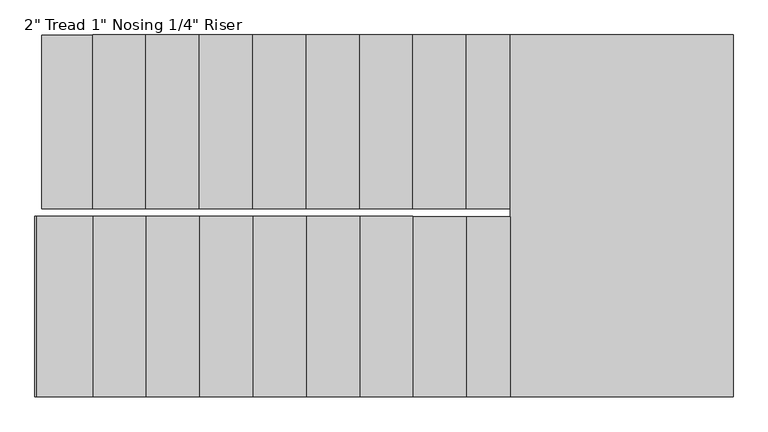
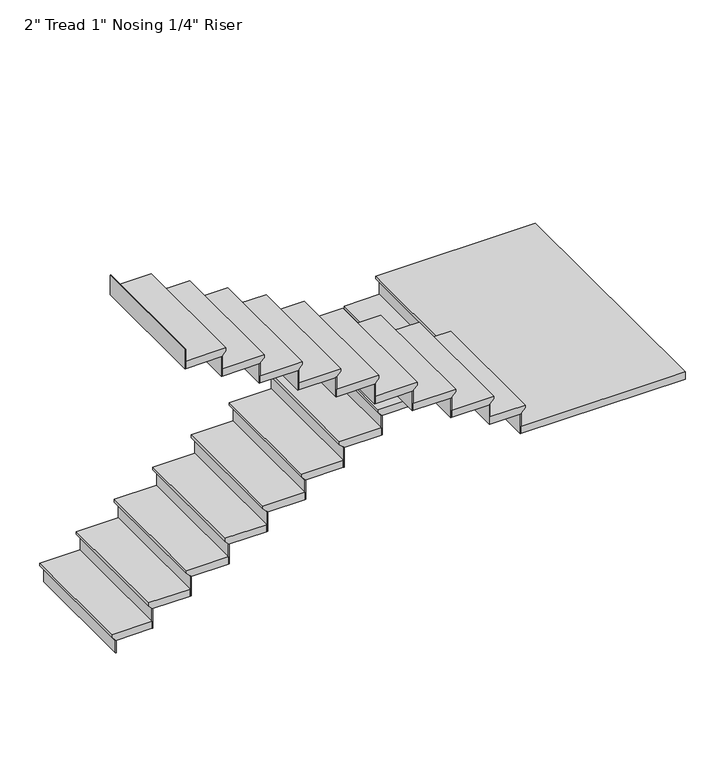
"""IFC4 building model written with IfcOpenShell, lengths in millimetres: stair flight geometry."""

from ifc_helpers import new_model, si_unit, origin, place, context, project, spatial, faceted_brep, source, transform, mapped, element, save


def stair_flight_04592867(model_context):
    return source(origin(), model_context, "Body", "Brep", [
        faceted_brep([(1537.1941283, 180.9547293, 3166.11), (1537.1941283, 180.9547293, 3185.16), (1537.1941283, 1006.4547293, 3185.16), (1537.1941283, 1006.4547293, 3166.11), (1562.5941283, 180.9547293, 3140.71), (1562.5941283, 1006.4547293, 3140.71), (1804.8381368, 180.9547293, 3185.16), (1804.8381368, 1006.4547293, 3185.16), (1562.5941283, 1006.4547293, 3134.36), (1804.8381368, 1006.4547293, 3134.36), (1804.8381368, 180.9547293, 3134.36), (1562.5941283, 180.9547293, 3134.36)], [[[0, 1, 2, 3]], [[4, 0, 3, 5]], [[2, 1, 6, 7]], [[8, 9, 10, 11]], [[2, 7, 9, 8, 5, 3]], [[8, 11, 4, 5]], [[6, 1, 0, 4, 11, 10]], [[7, 6, 10, 9]]]),
        faceted_brep([(1562.5941283, 180.9547293, 3134.36), (1562.5941283, 180.9547293, 3048.0), (1568.9441283, 180.9547293, 3048.0), (1568.9441283, 180.9547293, 3134.36), (1562.5941283, 1006.4547293, 3134.36), (1568.9441283, 1006.4547293, 3134.36), (1568.9441283, 1006.4547293, 3048.0), (1562.5941283, 1006.4547293, 3048.0)], [[[0, 1, 2, 3]], [[4, 5, 6, 7]], [[1, 0, 4, 7]], [[2, 1, 7, 6]], [[3, 2, 6, 5]], [[0, 3, 5, 4]]]),
        faceted_brep([(1804.8381368, 180.9547293, 3271.52), (1804.8381368, 180.9547293, 3134.36), (1811.1881368, 180.9547293, 3134.36), (1811.1881368, 180.9547293, 3271.52), (1804.8381368, 1006.4547293, 3271.52), (1811.1881368, 1006.4547293, 3271.52), (1811.1881368, 1006.4547293, 3134.36), (1804.8381368, 1006.4547293, 3134.36)], [[[0, 1, 2, 3]], [[4, 5, 6, 7]], [[1, 0, 4, 7]], [[2, 1, 7, 6]], [[3, 2, 6, 5]], [[0, 3, 5, 4]]]),
        faceted_brep([(1779.4381368, 1006.4547293, 3322.32), (1779.4381368, 180.9547293, 3322.32), (2058.8381368, 180.9547293, 3322.32), (2058.8381368, 1006.4547293, 3322.32), (1804.8381368, 1006.4547293, 3271.52), (2058.8381368, 1006.4547293, 3271.52), (2058.8381368, 180.9547293, 3271.52), (1804.8381368, 180.9547293, 3271.52), (1804.8381368, 1006.4547293, 3277.87), (1779.4381368, 1006.4547293, 3303.27), (1804.8381368, 180.9547293, 3277.87), (1779.4381368, 180.9547293, 3303.27)], [[[0, 1, 2, 3]], [[4, 5, 6, 7]], [[0, 3, 5, 4, 8, 9]], [[4, 7, 10, 8]], [[2, 1, 11, 10, 7, 6]], [[3, 2, 6, 5]], [[11, 1, 0, 9]], [[10, 11, 9, 8]]]),
        faceted_brep([(2058.8381368, 180.9547293, 3408.68), (2058.8381368, 180.9547293, 3271.52), (2065.1881368, 180.9547293, 3271.52), (2065.1881368, 180.9547293, 3408.68), (2058.8381368, 1006.4547293, 3408.68), (2065.1881368, 1006.4547293, 3408.68), (2065.1881368, 1006.4547293, 3271.52), (2058.8381368, 1006.4547293, 3271.52)], [[[0, 1, 2, 3]], [[4, 5, 6, 7]], [[1, 0, 4, 7]], [[2, 1, 7, 6]], [[3, 2, 6, 5]], [[0, 3, 5, 4]]]),
        faceted_brep([(2033.4381368, 1006.4547293, 3459.48), (2033.4381368, 180.9547293, 3459.48), (2312.8381368, 180.9547293, 3459.48), (2312.8381368, 1006.4547293, 3459.48), (2058.8381368, 1006.4547293, 3408.68), (2312.8381368, 1006.4547293, 3408.68), (2312.8381368, 180.9547293, 3408.68), (2058.8381368, 180.9547293, 3408.68), (2058.8381368, 1006.4547293, 3415.03), (2033.4381368, 1006.4547293, 3440.43), (2058.8381368, 180.9547293, 3415.03), (2033.4381368, 180.9547293, 3440.43)], [[[0, 1, 2, 3]], [[4, 5, 6, 7]], [[0, 3, 5, 4, 8, 9]], [[4, 7, 10, 8]], [[2, 1, 11, 10, 7, 6]], [[3, 2, 6, 5]], [[11, 1, 0, 9]], [[10, 11, 9, 8]]]),
        faceted_brep([(2312.8381368, 180.9547293, 3545.84), (2312.8381368, 180.9547293, 3408.68), (2319.1881368, 180.9547293, 3408.68), (2319.1881368, 180.9547293, 3545.84), (2312.8381368, 1006.4547293, 3545.84), (2319.1881368, 1006.4547293, 3545.84), (2319.1881368, 1006.4547293, 3408.68), (2312.8381368, 1006.4547293, 3408.68)], [[[0, 1, 2, 3]], [[4, 5, 6, 7]], [[1, 0, 4, 7]], [[2, 1, 7, 6]], [[3, 2, 6, 5]], [[0, 3, 5, 4]]]),
        faceted_brep([(2287.4381368, 1006.4547293, 3596.64), (2287.4381368, 180.9547293, 3596.64), (2566.8381368, 180.9547293, 3596.64), (2566.8381368, 1006.4547293, 3596.64), (2312.8381368, 1006.4547293, 3545.84), (2566.8381368, 1006.4547293, 3545.84), (2566.8381368, 180.9547293, 3545.84), (2312.8381368, 180.9547293, 3545.84), (2312.8381368, 1006.4547293, 3552.19), (2287.4381368, 1006.4547293, 3577.59), (2312.8381368, 180.9547293, 3552.19), (2287.4381368, 180.9547293, 3577.59)], [[[0, 1, 2, 3]], [[4, 5, 6, 7]], [[0, 3, 5, 4, 8, 9]], [[4, 7, 10, 8]], [[2, 1, 11, 10, 7, 6]], [[3, 2, 6, 5]], [[11, 1, 0, 9]], [[10, 11, 9, 8]]]),
        faceted_brep([(2566.8381368, 180.9547293, 3683.0), (2566.8381368, 180.9547293, 3545.84), (2573.1881368, 180.9547293, 3545.84), (2573.1881368, 180.9547293, 3683.0), (2566.8381368, 1006.4547293, 3683.0), (2573.1881368, 1006.4547293, 3683.0), (2573.1881368, 1006.4547293, 3545.84), (2566.8381368, 1006.4547293, 3545.84)], [[[0, 1, 2, 3]], [[4, 5, 6, 7]], [[1, 0, 4, 7]], [[2, 1, 7, 6]], [[3, 2, 6, 5]], [[0, 3, 5, 4]]]),
        faceted_brep([(2541.4381368, 1006.4547293, 3733.8), (2541.4381368, 180.9547293, 3733.8), (2820.8381368, 180.9547293, 3733.8), (2820.8381368, 1006.4547293, 3733.8), (2566.8381368, 1006.4547293, 3683.0), (2820.8381368, 1006.4547293, 3683.0), (2820.8381368, 180.9547293, 3683.0), (2566.8381368, 180.9547293, 3683.0), (2566.8381368, 1006.4547293, 3689.35), (2541.4381368, 1006.4547293, 3714.75), (2566.8381368, 180.9547293, 3689.35), (2541.4381368, 180.9547293, 3714.75)], [[[0, 1, 2, 3]], [[4, 5, 6, 7]], [[0, 3, 5, 4, 8, 9]], [[4, 7, 10, 8]], [[2, 1, 11, 10, 7, 6]], [[3, 2, 6, 5]], [[11, 1, 0, 9]], [[10, 11, 9, 8]]]),
        faceted_brep([(2820.8381368, 180.9547293, 3820.16), (2820.8381368, 180.9547293, 3683.0), (2827.1881368, 180.9547293, 3683.0), (2827.1881368, 180.9547293, 3820.16), (2820.8381368, 1006.4547293, 3820.16), (2827.1881368, 1006.4547293, 3820.16), (2827.1881368, 1006.4547293, 3683.0), (2820.8381368, 1006.4547293, 3683.0)], [[[0, 1, 2, 3]], [[4, 5, 6, 7]], [[1, 0, 4, 7]], [[2, 1, 7, 6]], [[3, 2, 6, 5]], [[0, 3, 5, 4]]]),
        faceted_brep([(2795.4381368, 1006.4547293, 3870.96), (2795.4381368, 180.9547293, 3870.96), (3074.8381368, 180.9547293, 3870.96), (3074.8381368, 1006.4547293, 3870.96), (2820.8381368, 1006.4547293, 3820.16), (3074.8381368, 1006.4547293, 3820.16), (3074.8381368, 180.9547293, 3820.16), (2820.8381368, 180.9547293, 3820.16), (2820.8381368, 1006.4547293, 3826.51), (2795.4381368, 1006.4547293, 3851.91), (2820.8381368, 180.9547293, 3826.51), (2795.4381368, 180.9547293, 3851.91)], [[[0, 1, 2, 3]], [[4, 5, 6, 7]], [[0, 3, 5, 4, 8, 9]], [[4, 7, 10, 8]], [[2, 1, 11, 10, 7, 6]], [[3, 2, 6, 5]], [[11, 1, 0, 9]], [[10, 11, 9, 8]]]),
        faceted_brep([(3074.8381368, 180.9547293, 3957.32), (3074.8381368, 180.9547293, 3820.16), (3081.1881368, 180.9547293, 3820.16), (3081.1881368, 180.9547293, 3957.32), (3074.8381368, 1006.4547293, 3957.32), (3081.1881368, 1006.4547293, 3957.32), (3081.1881368, 1006.4547293, 3820.16), (3074.8381368, 1006.4547293, 3820.16)], [[[0, 1, 2, 3]], [[4, 5, 6, 7]], [[1, 0, 4, 7]], [[2, 1, 7, 6]], [[3, 2, 6, 5]], [[0, 3, 5, 4]]]),
        faceted_brep([(3049.4381368, 1006.4547293, 4008.12), (3049.4381368, 180.9547293, 4008.12), (3328.8381368, 180.9547293, 4008.12), (3328.8381368, 1006.4547293, 4008.12), (3074.8381368, 1006.4547293, 3957.32), (3328.8381368, 1006.4547293, 3957.32), (3328.8381368, 180.9547293, 3957.32), (3074.8381368, 180.9547293, 3957.32), (3074.8381368, 1006.4547293, 3963.67), (3049.4381368, 1006.4547293, 3989.07), (3074.8381368, 180.9547293, 3963.67), (3049.4381368, 180.9547293, 3989.07)], [[[0, 1, 2, 3]], [[4, 5, 6, 7]], [[0, 3, 5, 4, 8, 9]], [[4, 7, 10, 8]], [[2, 1, 11, 10, 7, 6]], [[3, 2, 6, 5]], [[11, 1, 0, 9]], [[10, 11, 9, 8]]]),
        faceted_brep([(3328.8381368, 180.9547293, 4094.48), (3328.8381368, 180.9547293, 3957.32), (3335.1881368, 180.9547293, 3957.32), (3335.1881368, 180.9547293, 4094.48), (3328.8381368, 1006.4547293, 4094.48), (3335.1881368, 1006.4547293, 4094.48), (3335.1881368, 1006.4547293, 3957.32), (3328.8381368, 1006.4547293, 3957.32)], [[[0, 1, 2, 3]], [[4, 5, 6, 7]], [[1, 0, 4, 7]], [[2, 1, 7, 6]], [[3, 2, 6, 5]], [[0, 3, 5, 4]]]),
        faceted_brep([(3303.4381368, 1006.4547293, 4145.28), (3303.4381368, 180.9547293, 4145.28), (3582.8381368, 180.9547293, 4145.28), (3582.8381368, 1006.4547293, 4145.28), (3328.8381368, 1006.4547293, 4094.48), (3582.8381368, 1006.4547293, 4094.48), (3582.8381368, 180.9547293, 4094.48), (3328.8381368, 180.9547293, 4094.48), (3328.8381368, 1006.4547293, 4100.83), (3303.4381368, 1006.4547293, 4126.23), (3328.8381368, 180.9547293, 4100.83), (3303.4381368, 180.9547293, 4126.23)], [[[0, 1, 2, 3]], [[4, 5, 6, 7]], [[0, 3, 5, 4, 8, 9]], [[4, 7, 10, 8]], [[2, 1, 11, 10, 7, 6]], [[3, 2, 6, 5]], [[11, 1, 0, 9]], [[10, 11, 9, 8]]]),
        faceted_brep([(3582.8381368, 180.9547293, 4231.64), (3582.8381368, 180.9547293, 4094.48), (3589.1881368, 180.9547293, 4094.48), (3589.1881368, 180.9547293, 4231.64), (3582.8381368, 1006.4547293, 4231.64), (3589.1881368, 1006.4547293, 4231.64), (3589.1881368, 1006.4547293, 4094.48), (3582.8381368, 1006.4547293, 4094.48)], [[[0, 1, 2, 3]], [[4, 5, 6, 7]], [[1, 0, 4, 7]], [[2, 1, 7, 6]], [[3, 2, 6, 5]], [[0, 3, 5, 4]]]),
        faceted_brep([(3557.4381368, 1006.4547293, 4282.44), (3557.4381368, 180.9547293, 4282.44), (3791.2648053, 180.9547293, 4282.44), (3791.2648053, 1006.4547293, 4282.44), (3582.8381368, 1006.4547293, 4231.64), (3791.2648053, 1006.4547293, 4231.64), (3791.2648053, 180.9547293, 4231.64), (3582.8381368, 180.9547293, 4231.64), (3582.8381368, 1006.4547293, 4237.99), (3557.4381368, 1006.4547293, 4263.39), (3582.8381368, 180.9547293, 4237.99), (3557.4381368, 180.9547293, 4263.39)], [[[0, 1, 2, 3]], [[4, 5, 6, 7]], [[0, 3, 5, 4, 8, 9]], [[4, 7, 10, 8]], [[2, 1, 11, 10, 7, 6]], [[3, 2, 6, 5]], [[11, 1, 0, 9]], [[10, 11, 9, 8]]]),
        faceted_brep([(3791.2648053, 180.9547293, 4368.8), (3791.2648053, 180.9547293, 4231.64), (3797.6148053, 180.9547293, 4231.64), (3797.6148053, 180.9547293, 4368.8), (3791.2648053, 1006.4547293, 4368.8), (3797.6148053, 1006.4547293, 4368.8), (3797.6148053, 1006.4547293, 4231.64), (3791.2648053, 1006.4547293, 4231.64)], [[[0, 1, 2, 3]], [[4, 5, 6, 7]], [[1, 0, 4, 7]], [[2, 1, 7, 6]], [[3, 2, 6, 5]], [[0, 3, 5, 4]]]),
        faceted_brep([(3740.4648053, -714.2964201, 4419.6), (4826.4941283, -714.2964201, 4419.6), (4826.4941283, 1006.4547293, 4419.6), (3765.8648053, 1006.4547293, 4419.6), (3765.8648053, 142.8547293, 4419.6), (3740.4648053, 142.8547293, 4419.6), (4826.4941283, -714.2964201, 4368.8), (3740.4648053, -714.2964201, 4368.8), (3740.4648053, 142.8547293, 4368.8), (3765.8648053, 142.8547293, 4368.8), (3765.8648053, 180.9547293, 4368.8), (3791.2648053, 180.9547293, 4368.8), (3791.2648053, 1006.4547293, 4368.8), (4826.4941283, 1006.4547293, 4368.8), (3791.2648053, 1006.4547293, 4375.15), (3765.8648053, 1006.4547293, 4400.55), (3791.2648053, 180.9547293, 4375.15), (3765.8648053, 180.9547293, 4400.55)], [[[0, 1, 2, 3, 4, 5]], [[6, 7, 8, 9, 10, 11, 12, 13]], [[1, 0, 7, 6]], [[2, 1, 6, 13]], [[3, 2, 13, 12, 14, 15]], [[12, 11, 16, 14]], [[11, 10, 17, 16]], [[4, 3, 15, 17, 10, 9]], [[5, 4, 9, 8]], [[0, 5, 8, 7]], [[15, 14, 16, 17]]]),
        faceted_brep([(3740.4648053, 142.8547293, 4505.96), (3740.4648053, 142.8547293, 4368.8), (3734.1148053, 142.8547293, 4368.8), (3734.1148053, 142.8547293, 4505.96), (3740.4648053, -714.2964201, 4505.96), (3734.1148053, -714.2964201, 4505.96), (3734.1148053, -714.2964201, 4368.8), (3740.4648053, -714.2964201, 4368.8)], [[[0, 1, 2, 3]], [[4, 5, 6, 7]], [[1, 0, 4, 7]], [[2, 1, 7, 6]], [[3, 2, 6, 5]], [[0, 3, 5, 4]]]),
        faceted_brep([(3765.8648053, -714.2964201, 4556.76), (3765.8648053, 142.8547293, 4556.76), (3532.0381368, 142.8547293, 4556.76), (3532.0381368, -714.2964201, 4556.76), (3740.4648053, -714.2964201, 4505.96), (3532.0381368, -714.2964201, 4505.96), (3532.0381368, 142.8547293, 4505.96), (3740.4648053, 142.8547293, 4505.96), (3740.4648053, -714.2964201, 4512.31), (3765.8648053, -714.2964201, 4537.71), (3740.4648053, 142.8547293, 4512.31), (3765.8648053, 142.8547293, 4537.71)], [[[0, 1, 2, 3]], [[4, 5, 6, 7]], [[0, 3, 5, 4, 8, 9]], [[4, 7, 10, 8]], [[2, 1, 11, 10, 7, 6]], [[3, 2, 6, 5]], [[11, 1, 0, 9]], [[10, 11, 9, 8]]]),
        faceted_brep([(3532.0381368, 142.8547293, 4643.12), (3532.0381368, 142.8547293, 4505.96), (3525.6881368, 142.8547293, 4505.96), (3525.6881368, 142.8547293, 4643.12), (3532.0381368, -714.2964201, 4643.12), (3525.6881368, -714.2964201, 4643.12), (3525.6881368, -714.2964201, 4505.96), (3532.0381368, -714.2964201, 4505.96)], [[[0, 1, 2, 3]], [[4, 5, 6, 7]], [[1, 0, 4, 7]], [[2, 1, 7, 6]], [[3, 2, 6, 5]], [[0, 3, 5, 4]]]),
        faceted_brep([(3557.4381368, -714.2964201, 4693.92), (3557.4381368, 142.8547293, 4693.92), (3278.0381368, 142.8547293, 4693.92), (3278.0381368, -714.2964201, 4693.92), (3532.0381368, -714.2964201, 4643.12), (3278.0381368, -714.2964201, 4643.12), (3278.0381368, 142.8547293, 4643.12), (3532.0381368, 142.8547293, 4643.12), (3532.0381368, -714.2964201, 4649.47), (3557.4381368, -714.2964201, 4674.87), (3532.0381368, 142.8547293, 4649.47), (3557.4381368, 142.8547293, 4674.87)], [[[0, 1, 2, 3]], [[4, 5, 6, 7]], [[0, 3, 5, 4, 8, 9]], [[4, 7, 10, 8]], [[2, 1, 11, 10, 7, 6]], [[3, 2, 6, 5]], [[11, 1, 0, 9]], [[10, 11, 9, 8]]]),
        faceted_brep([(3278.0381368, 142.8547293, 4780.28), (3278.0381368, 142.8547293, 4643.12), (3271.6881368, 142.8547293, 4643.12), (3271.6881368, 142.8547293, 4780.28), (3278.0381368, -714.2964201, 4780.28), (3271.6881368, -714.2964201, 4780.28), (3271.6881368, -714.2964201, 4643.12), (3278.0381368, -714.2964201, 4643.12)], [[[0, 1, 2, 3]], [[4, 5, 6, 7]], [[1, 0, 4, 7]], [[2, 1, 7, 6]], [[3, 2, 6, 5]], [[0, 3, 5, 4]]]),
        faceted_brep([(3303.4381368, -714.2964201, 4831.08), (3303.4381368, 142.8547293, 4831.08), (3024.0381368, 142.8547293, 4831.08), (3024.0381368, -714.2964201, 4831.08), (3278.0381368, -714.2964201, 4780.28), (3024.0381368, -714.2964201, 4780.28), (3024.0381368, 142.8547293, 4780.28), (3278.0381368, 142.8547293, 4780.28), (3278.0381368, -714.2964201, 4786.63), (3303.4381368, -714.2964201, 4812.03), (3278.0381368, 142.8547293, 4786.63), (3303.4381368, 142.8547293, 4812.03)], [[[0, 1, 2, 3]], [[4, 5, 6, 7]], [[0, 3, 5, 4, 8, 9]], [[4, 7, 10, 8]], [[2, 1, 11, 10, 7, 6]], [[3, 2, 6, 5]], [[11, 1, 0, 9]], [[10, 11, 9, 8]]]),
        faceted_brep([(3024.0381368, 142.8547293, 4917.44), (3024.0381368, 142.8547293, 4780.28), (3017.6881368, 142.8547293, 4780.28), (3017.6881368, 142.8547293, 4917.44), (3024.0381368, -714.2964201, 4917.44), (3017.6881368, -714.2964201, 4917.44), (3017.6881368, -714.2964201, 4780.28), (3024.0381368, -714.2964201, 4780.28)], [[[0, 1, 2, 3]], [[4, 5, 6, 7]], [[1, 0, 4, 7]], [[2, 1, 7, 6]], [[3, 2, 6, 5]], [[0, 3, 5, 4]]]),
        faceted_brep([(3049.4381368, -714.2964201, 4968.24), (3049.4381368, 142.8547293, 4968.24), (2770.0381368, 142.8547293, 4968.24), (2770.0381368, -714.2964201, 4968.24), (3024.0381368, -714.2964201, 4917.44), (2770.0381368, -714.2964201, 4917.44), (2770.0381368, 142.8547293, 4917.44), (3024.0381368, 142.8547293, 4917.44), (3024.0381368, -714.2964201, 4923.79), (3049.4381368, -714.2964201, 4949.19), (3024.0381368, 142.8547293, 4923.79), (3049.4381368, 142.8547293, 4949.19)], [[[0, 1, 2, 3]], [[4, 5, 6, 7]], [[0, 3, 5, 4, 8, 9]], [[4, 7, 10, 8]], [[2, 1, 11, 10, 7, 6]], [[3, 2, 6, 5]], [[11, 1, 0, 9]], [[10, 11, 9, 8]]]),
        faceted_brep([(2770.0381368, 142.8547293, 5054.6), (2770.0381368, 142.8547293, 4917.44), (2763.6881368, 142.8547293, 4917.44), (2763.6881368, 142.8547293, 5054.6), (2770.0381368, -714.2964201, 5054.6), (2763.6881368, -714.2964201, 5054.6), (2763.6881368, -714.2964201, 4917.44), (2770.0381368, -714.2964201, 4917.44)], [[[0, 1, 2, 3]], [[4, 5, 6, 7]], [[1, 0, 4, 7]], [[2, 1, 7, 6]], [[3, 2, 6, 5]], [[0, 3, 5, 4]]]),
        faceted_brep([(2795.4381368, -714.2964201, 5105.4), (2795.4381368, 142.8547293, 5105.4), (2516.0381368, 142.8547293, 5105.4), (2516.0381368, -714.2964201, 5105.4), (2770.0381368, -714.2964201, 5054.6), (2516.0381368, -714.2964201, 5054.6), (2516.0381368, 142.8547293, 5054.6), (2770.0381368, 142.8547293, 5054.6), (2770.0381368, -714.2964201, 5060.95), (2795.4381368, -714.2964201, 5086.35), (2770.0381368, 142.8547293, 5060.95), (2795.4381368, 142.8547293, 5086.35)], [[[0, 1, 2, 3]], [[4, 5, 6, 7]], [[0, 3, 5, 4, 8, 9]], [[4, 7, 10, 8]], [[2, 1, 11, 10, 7, 6]], [[3, 2, 6, 5]], [[11, 1, 0, 9]], [[10, 11, 9, 8]]]),
        faceted_brep([(2516.0381368, 142.8547293, 5191.76), (2516.0381368, 142.8547293, 5054.6), (2509.6881368, 142.8547293, 5054.6), (2509.6881368, 142.8547293, 5191.76), (2516.0381368, -714.2964201, 5191.76), (2509.6881368, -714.2964201, 5191.76), (2509.6881368, -714.2964201, 5054.6), (2516.0381368, -714.2964201, 5054.6)], [[[0, 1, 2, 3]], [[4, 5, 6, 7]], [[1, 0, 4, 7]], [[2, 1, 7, 6]], [[3, 2, 6, 5]], [[0, 3, 5, 4]]]),
        faceted_brep([(2541.4381368, -714.2964201, 5242.56), (2541.4381368, 142.8547293, 5242.56), (2262.0381368, 142.8547293, 5242.56), (2262.0381368, -714.2964201, 5242.56), (2516.0381368, -714.2964201, 5191.76), (2262.0381368, -714.2964201, 5191.76), (2262.0381368, 142.8547293, 5191.76), (2516.0381368, 142.8547293, 5191.76), (2516.0381368, -714.2964201, 5198.11), (2541.4381368, -714.2964201, 5223.51), (2516.0381368, 142.8547293, 5198.11), (2541.4381368, 142.8547293, 5223.51)], [[[0, 1, 2, 3]], [[4, 5, 6, 7]], [[0, 3, 5, 4, 8, 9]], [[4, 7, 10, 8]], [[2, 1, 11, 10, 7, 6]], [[3, 2, 6, 5]], [[11, 1, 0, 9]], [[10, 11, 9, 8]]]),
        faceted_brep([(2262.0381368, 142.8547293, 5328.92), (2262.0381368, 142.8547293, 5191.76), (2255.6881368, 142.8547293, 5191.76), (2255.6881368, 142.8547293, 5328.92), (2262.0381368, -714.2964201, 5328.92), (2255.6881368, -714.2964201, 5328.92), (2255.6881368, -714.2964201, 5191.76), (2262.0381368, -714.2964201, 5191.76)], [[[0, 1, 2, 3]], [[4, 5, 6, 7]], [[1, 0, 4, 7]], [[2, 1, 7, 6]], [[3, 2, 6, 5]], [[0, 3, 5, 4]]]),
        faceted_brep([(2287.4381368, -714.2964201, 5379.72), (2287.4381368, 142.8547293, 5379.72), (2008.0381368, 142.8547293, 5379.72), (2008.0381368, -714.2964201, 5379.72), (2262.0381368, -714.2964201, 5328.92), (2008.0381368, -714.2964201, 5328.92), (2008.0381368, 142.8547293, 5328.92), (2262.0381368, 142.8547293, 5328.92), (2262.0381368, -714.2964201, 5335.27), (2287.4381368, -714.2964201, 5360.67), (2262.0381368, 142.8547293, 5335.27), (2287.4381368, 142.8547293, 5360.67)], [[[0, 1, 2, 3]], [[4, 5, 6, 7]], [[0, 3, 5, 4, 8, 9]], [[4, 7, 10, 8]], [[2, 1, 11, 10, 7, 6]], [[3, 2, 6, 5]], [[11, 1, 0, 9]], [[10, 11, 9, 8]]]),
        faceted_brep([(2008.0381368, 142.8547293, 5466.08), (2008.0381368, 142.8547293, 5328.92), (2001.6881368, 142.8547293, 5328.92), (2001.6881368, 142.8547293, 5466.08), (2008.0381368, -714.2964201, 5466.08), (2001.6881368, -714.2964201, 5466.08), (2001.6881368, -714.2964201, 5328.92), (2008.0381368, -714.2964201, 5328.92)], [[[0, 1, 2, 3]], [[4, 5, 6, 7]], [[1, 0, 4, 7]], [[2, 1, 7, 6]], [[3, 2, 6, 5]], [[0, 3, 5, 4]]]),
        faceted_brep([(2033.4381368, -714.2964201, 5516.88), (2033.4381368, 142.8547293, 5516.88), (1754.0381368, 142.8547293, 5516.88), (1754.0381368, -714.2964201, 5516.88), (2008.0381368, -714.2964201, 5466.08), (1754.0381368, -714.2964201, 5466.08), (1754.0381368, 142.8547293, 5466.08), (2008.0381368, 142.8547293, 5466.08), (2008.0381368, -714.2964201, 5472.43), (2033.4381368, -714.2964201, 5497.83), (2008.0381368, 142.8547293, 5472.43), (2033.4381368, 142.8547293, 5497.83)], [[[0, 1, 2, 3]], [[4, 5, 6, 7]], [[0, 3, 5, 4, 8, 9]], [[4, 7, 10, 8]], [[2, 1, 11, 10, 7, 6]], [[3, 2, 6, 5]], [[11, 1, 0, 9]], [[10, 11, 9, 8]]]),
        faceted_brep([(1754.0381368, 142.8547293, 5603.24), (1754.0381368, 142.8547293, 5466.08), (1747.6881368, 142.8547293, 5466.08), (1747.6881368, 142.8547293, 5603.24), (1754.0381368, -714.2964201, 5603.24), (1747.6881368, -714.2964201, 5603.24), (1747.6881368, -714.2964201, 5466.08), (1754.0381368, -714.2964201, 5466.08)], [[[0, 1, 2, 3]], [[4, 5, 6, 7]], [[1, 0, 4, 7]], [[2, 1, 7, 6]], [[3, 2, 6, 5]], [[0, 3, 5, 4]]]),
        faceted_brep([(1511.7941283, 142.8547293, 5740.4), (1511.7941283, 142.8547293, 5603.24), (1505.4441283, 142.8547293, 5603.24), (1505.4441283, 142.8547293, 5740.4), (1511.7941283, -714.2964201, 5740.4), (1505.4441283, -714.2964201, 5740.4), (1505.4441283, -714.2964201, 5603.24), (1511.7941283, -714.2964201, 5603.24)], [[[0, 1, 2, 3]], [[4, 5, 6, 7]], [[1, 0, 4, 7]], [[2, 1, 7, 6]], [[3, 2, 6, 5]], [[0, 3, 5, 4]]]),
        faceted_brep([(1779.4381368, -714.2964201, 5654.04), (1779.4381368, 142.8547293, 5654.04), (1511.7941283, 142.8547293, 5654.04), (1511.7941283, -714.2964201, 5654.04), (1754.0381368, -714.2964201, 5603.24), (1511.7941283, -714.2964201, 5603.24), (1511.7941283, 142.8547293, 5603.24), (1754.0381368, 142.8547293, 5603.24), (1754.0381368, -714.2964201, 5609.59), (1779.4381368, -714.2964201, 5634.99), (1754.0381368, 142.8547293, 5609.59), (1779.4381368, 142.8547293, 5634.99)], [[[0, 1, 2, 3]], [[4, 5, 6, 7]], [[0, 3, 5, 4, 8, 9]], [[4, 7, 10, 8]], [[2, 1, 11, 10, 7, 6]], [[3, 2, 6, 5]], [[11, 1, 0, 9]], [[10, 11, 9, 8]]]),
    ])


if __name__ == "__main__":
    model = new_model("IFC4")
    model_context = context("Model", 3, world=origin())
    ifc_project = project(units=[si_unit("LENGTHUNIT", "METRE", prefix="MILLI")], contexts=[model_context])
    site = spatial("IfcSite", under=ifc_project)
    building = spatial("IfcBuilding", under=site)
    placement = place(None, origin())
    stair_flight_shape = stair_flight_04592867(model_context)
    element("IfcStairFlight", 1, ObjectType="2\" Tread 1\" Nosing 1/4\" Riser", at=placement, inside=building, context=model_context, shape_type="MappedRepresentation", body=[
        mapped(stair_flight_shape, transform((0.0, 0.0, 0.0), x_axis=(1.0, 0.0, 0.0), y_axis=(0.0, 1.0, 0.0), z_axis=(0.0, 0.0, 1.0))),
    ])
    save(model, "model.ifc")
